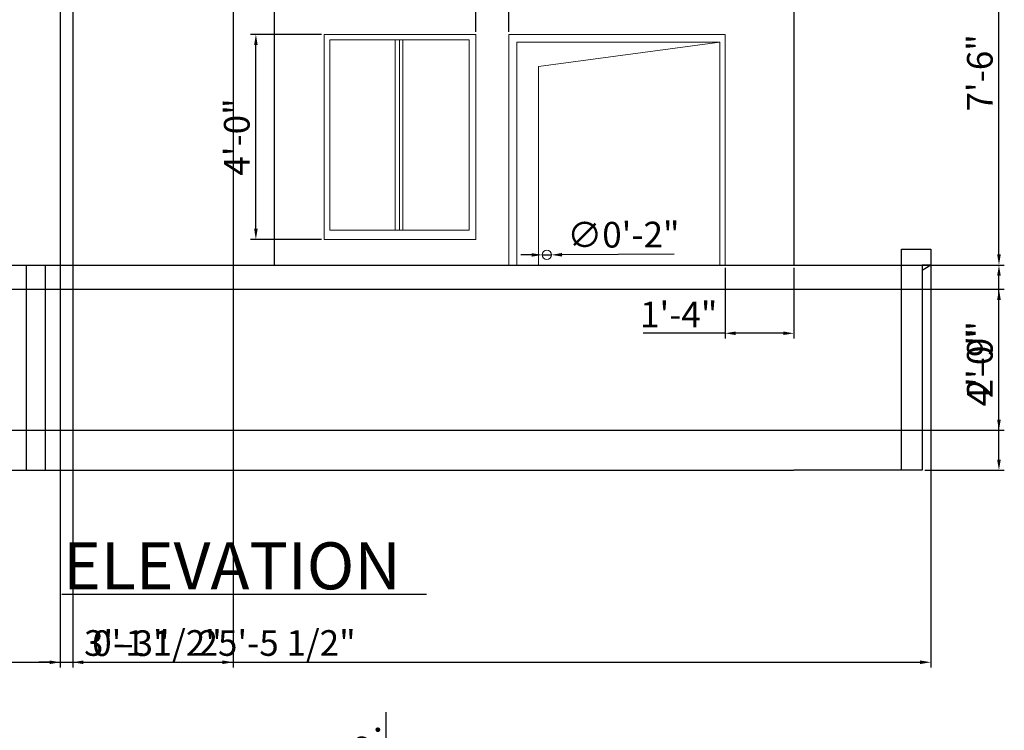
# Model space of a CAD drawing. Units: inches. Extents: x 2656 to 9931, y 1941 to 3068.
# Tile 29 of 46: x 2817 to 3047, y 2689 to 2855. Entities that reach past the tile are written whole.
import ezdxf

# ---------------------------------------------------------------- set-up
doc = ezdxf.new("R2010")
doc.units = ezdxf.units.IN
for name, color, linetype, lineweight in [('A-ANNO-DIMS', 2, 'Continuous', 18), ('A-ANNO-TEXT', 7, 'Continuous', 25), ('A-DOOR', 3, 'Continuous', 18), ('A-ELEV', 7, 'Continuous', 25), ('A-GLAZ', 4, 'Continuous', 18)]:
    doc.layers.add(name, color=color, linetype=linetype, lineweight=lineweight)
doc.styles.get("Standard").update_dxf_attribs({"font": 'arial.ttf'})
doc.dimstyles.new('ISO-25', dxfattribs={"dimtxt": 6, "dimasz": 2.5, "dimexe": 1.25, "dimexo": 0.625, "dimtad": 1, "dimdec": 0, "dimlunit": 3, "dimtxsty": 'Standard', "dimcen": 2.5, "dimadec": 0, "dimazin": 0, "dimtfac": 1, "dimtdec": 0, "dimtmove": 0, "dimatfit": 3, "dimfxl": 1, "dimarcsym": 0})

# ---------------------------------------------------------------- blocks, each defined once
blk = doc.blocks.new('*D33')
at = {"layer": 'A-ANNO-DIMS', "color": 0, "lineweight": -2, "transparency": 16777216}
for p, q in [((2902.86, 2595), (2902.86, 2693.32)), ((2899.03, 2595), (2904.11, 2595)), ((2902.86, 2567.84), (2902.86, 2592.5)), ((2899.03, 2565.34), (2904.11, 2565.34))]:
    blk.add_line(p, q, dxfattribs=at)
at = {"layer": 'A-ANNO-DIMS', "color": 0, "transparency": 16777216}
for points in [[(2902.44, 2592.5), (2903.27, 2592.5), (2902.86, 2595)], [(2902.44, 2567.84), (2903.27, 2567.84), (2902.86, 2565.34)]]:
    blk.add_solid(points, dxfattribs=at)
at = {"layer": 'Defpoints', "color": 0, "transparency": 16777216}
for p in [(2898.41, 2595), (2902.86, 2595), (2898.41, 2565.34)]:
    blk.add_point(p, dxfattribs=at)
at = {"layer": 'A-ANNO-DIMS', "color": 0, "transparency": 16777216, "insert": (2899.13, 2645.41), "char_height": 6, "attachment_point": 5, "rotation": 90}
blk.add_mtext('WC DOOR 2\'-5 1/2" TYP.', dxfattribs=at)
blk = doc.blocks.new('*D63')
at = {"layer": 'A-ANNO-DIMS', "color": 0, "lineweight": -2, "transparency": 16777216}
for p, q in [((2807.09, 2803.32), (2807.09, 2893)), ((2799.7, 2803.32), (2808.34, 2803.32)), ((2807.09, 2752.39), (2807.09, 2800.82)), ((2799.7, 2749.89), (2808.34, 2749.89))]:
    blk.add_line(p, q, dxfattribs=at)
at = {"layer": 'A-ANNO-DIMS', "color": 0, "transparency": 16777216}
for points in [[(2806.67, 2800.82), (2807.5, 2800.82), (2807.09, 2803.32)], [(2806.67, 2752.39), (2807.5, 2752.39), (2807.09, 2749.89)]]:
    blk.add_solid(points, dxfattribs=at)
at = {"layer": 'Defpoints', "color": 0, "transparency": 16777216}
for p in [(2799.07, 2803.32), (2807.09, 2803.32), (2799.07, 2749.89)]:
    blk.add_point(p, dxfattribs=at)
at = {"layer": 'A-ANNO-DIMS', "color": 0, "transparency": 16777216, "insert": (2803.36, 2849.41), "char_height": 6, "attachment_point": 5, "rotation": 90}
blk.add_mtext('FRONT GATE 4\'-5 1/2"', dxfattribs=at)
blk = doc.blocks.new('*D77')
at = {"layer": 'A-ANNO-DIMS', "color": 0, "lineweight": -2, "transparency": 16777216}
for p, q in [((2724.52, 2799.77), (2724.52, 2703.71)), ((3030.16, 2801), (3030.16, 2703.71)), ((2727.02, 2704.96), (3027.66, 2704.96))]:
    blk.add_line(p, q, dxfattribs=at)
at = {"layer": 'A-ANNO-DIMS', "color": 0, "transparency": 16777216}
for points in [[(2727.02, 2705.38), (2727.02, 2704.54), (2724.52, 2704.96)], [(3027.66, 2705.38), (3027.66, 2704.54), (3030.16, 2704.96)]]:
    blk.add_solid(points, dxfattribs=at)
at = {"layer": 'Defpoints', "color": 0, "transparency": 16777216}
for p in [(2724.52, 2800.4), (3030.16, 2801.62), (3030.16, 2704.96)]:
    blk.add_point(p, dxfattribs=at)
at = {"layer": 'A-ANNO-DIMS', "color": 0, "transparency": 16777216, "insert": (2877.34, 2708.69), "char_height": 6, "attachment_point": 5}
blk.add_mtext('25\'-5 1/2"', dxfattribs=at)
blk = doc.blocks.new('*D79')
at = {"layer": 'A-ANNO-DIMS', "color": 0, "lineweight": -2, "transparency": 16777216}
for p, q in [((3023.97, 2797.89), (3047.36, 2797.89)), ((3046.11, 2752.39), (3046.11, 2795.39)), ((3028.78, 2749.89), (3047.36, 2749.89))]:
    blk.add_line(p, q, dxfattribs=at)
at = {"layer": 'A-ANNO-DIMS', "color": 0, "transparency": 16777216}
for points in [[(3045.69, 2795.39), (3046.53, 2795.39), (3046.11, 2797.89)], [(3045.69, 2752.39), (3046.53, 2752.39), (3046.11, 2749.89)]]:
    blk.add_solid(points, dxfattribs=at)
at = {"layer": 'Defpoints', "color": 0, "transparency": 16777216}
for p in [(3023.35, 2797.89), (3046.11, 2797.89), (3028.16, 2749.89)]:
    blk.add_point(p, dxfattribs=at)
at = {"layer": 'A-ANNO-DIMS', "color": 0, "transparency": 16777216, "insert": (3042.42, 2773.89), "char_height": 6, "attachment_point": 5, "rotation": 90}
blk.add_mtext('4\'-0"', dxfattribs=at)
blk = doc.blocks.new('*D80')
at = {"layer": 'A-ANNO-DIMS', "color": 0, "lineweight": -2, "transparency": 16777216}
for p, q in [((3015.61, 2887.89), (3047.36, 2887.89)), ((3046.11, 2800.39), (3046.11, 2885.39)), ((2998.78, 2797.89), (3047.36, 2797.89))]:
    blk.add_line(p, q, dxfattribs=at)
at = {"layer": 'A-ANNO-DIMS', "color": 0, "transparency": 16777216}
for points in [[(3045.69, 2885.39), (3046.53, 2885.39), (3046.11, 2887.89)], [(3045.69, 2800.39), (3046.53, 2800.39), (3046.11, 2797.89)]]:
    blk.add_solid(points, dxfattribs=at)
at = {"layer": 'Defpoints', "color": 0, "transparency": 16777216}
for p in [(3014.98, 2887.89), (3046.11, 2887.89), (2998.16, 2797.89)]:
    blk.add_point(p, dxfattribs=at)
at = {"layer": 'A-ANNO-DIMS', "color": 0, "transparency": 16777216, "insert": (3042.42, 2842.89), "char_height": 6, "attachment_point": 5, "rotation": 90}
blk.add_mtext('7\'-6"', dxfattribs=at)
blk = doc.blocks.new('*D82')
at = {"layer": 'A-ANNO-DIMS', "color": 0, "lineweight": -2, "transparency": 16777216}
for p, q in [((2887.7, 2851.89), (2871.12, 2851.89)), ((2872.37, 2806.39), (2872.37, 2849.39)), ((2887.7, 2803.89), (2871.12, 2803.89))]:
    blk.add_line(p, q, dxfattribs=at)
at = {"layer": 'A-ANNO-DIMS', "color": 0, "transparency": 16777216}
for points in [[(2871.96, 2849.39), (2872.79, 2849.39), (2872.37, 2851.89)], [(2871.96, 2806.39), (2872.79, 2806.39), (2872.37, 2803.89)]]:
    blk.add_solid(points, dxfattribs=at)
at = {"layer": 'Defpoints', "color": 0, "transparency": 16777216}
for p in [(2872.37, 2851.89), (2888.32, 2851.89), (2888.32, 2803.89)]:
    blk.add_point(p, dxfattribs=at)
at = {"layer": 'A-ANNO-DIMS', "color": 0, "transparency": 16777216, "insert": (2868.68, 2827.89), "char_height": 6, "attachment_point": 5, "rotation": 90}
blk.add_mtext('4\'-0"', dxfattribs=at)
blk = doc.blocks.new('*D86')
at = {"layer": 'A-ANNO-DIMS', "color": 0, "lineweight": -2, "transparency": 16777216}
for p, q in [((2923.8, 2852.52), (2923.8, 2869.09)), ((2931.54, 2852.52), (2931.54, 2869.09)), ((2926.3, 2867.84), (2929.04, 2867.84)), ((2931.54, 2867.84), (2965.22, 2867.84))]:
    blk.add_line(p, q, dxfattribs=at)
at = {"layer": 'A-ANNO-DIMS', "color": 0, "transparency": 16777216}
for points in [[(2926.3, 2868.26), (2926.3, 2867.43), (2923.8, 2867.84)], [(2929.04, 2868.26), (2929.04, 2867.43), (2931.54, 2867.84)]]:
    blk.add_solid(points, dxfattribs=at)
at = {"layer": 'Defpoints', "color": 0, "transparency": 16777216}
for p in [(2931.54, 2867.84), (2923.8, 2851.89), (2931.54, 2851.89)]:
    blk.add_point(p, dxfattribs=at)
at = {"layer": 'A-ANNO-DIMS', "color": 0, "transparency": 16777216, "insert": (2949.63, 2871.57), "char_height": 6, "attachment_point": 5}
blk.add_mtext('0\'-7 1/2"', dxfattribs=at)
blk = doc.blocks.new('*D87')
at = {"layer": 'A-ANNO-DIMS', "color": 0, "lineweight": -2, "transparency": 16777216}
for p, q in [((2982.06, 2797.27), (2982.06, 2780.69)), ((2998.16, 2797.27), (2998.16, 2780.69)), ((2982.06, 2781.94), (2962.92, 2781.94)), ((2995.66, 2781.94), (2984.56, 2781.94))]:
    blk.add_line(p, q, dxfattribs=at)
at = {"layer": 'A-ANNO-DIMS', "color": 0, "transparency": 16777216}
for points in [[(2984.56, 2782.36), (2984.56, 2781.53), (2982.06, 2781.94)], [(2995.66, 2782.36), (2995.66, 2781.53), (2998.16, 2781.94)]]:
    blk.add_solid(points, dxfattribs=at)
at = {"layer": 'Defpoints', "color": 0, "transparency": 16777216}
for p in [(2982.06, 2797.89), (2998.16, 2797.89), (2982.06, 2781.94)]:
    blk.add_point(p, dxfattribs=at)
at = {"layer": 'A-ANNO-DIMS', "color": 0, "transparency": 16777216, "insert": (2971.24, 2785.58), "char_height": 6, "attachment_point": 5}
blk.add_mtext('1\'-4"', dxfattribs=at)
blk = doc.blocks.new('*D151')
at = {"layer": 'A-ANNO-DIMS', "color": 0, "lineweight": -2, "transparency": 16777216}
for p, q in [((2829.55, 2956.42), (2829.55, 2703.71)), ((2867.06, 2955.98), (2867.06, 2703.71)), ((2832.05, 2704.96), (2864.56, 2704.96))]:
    blk.add_line(p, q, dxfattribs=at)
at = {"layer": 'A-ANNO-DIMS', "color": 0, "transparency": 16777216}
for points in [[(2832.05, 2705.38), (2832.05, 2704.54), (2829.55, 2704.96)], [(2864.56, 2705.38), (2864.56, 2704.54), (2867.06, 2704.96)]]:
    blk.add_solid(points, dxfattribs=at)
at = {"layer": 'Defpoints', "color": 0, "transparency": 16777216}
for p in [(2829.55, 2957.05), (2867.06, 2956.61), (2867.06, 2704.96)]:
    blk.add_point(p, dxfattribs=at)
at = {"layer": 'A-ANNO-DIMS', "color": 0, "transparency": 16777216, "insert": (2848.3, 2708.69), "char_height": 6, "attachment_point": 5}
blk.add_mtext('3\'-1 1/2"', dxfattribs=at)
blk = doc.blocks.new('*D153')
at = {"layer": 'A-ANNO-DIMS', "color": 0, "lineweight": -2, "transparency": 16777216}
for p, q in [((2826.64, 2993.72), (2826.64, 2703.71)), ((2829.55, 2956.42), (2829.55, 2703.71)), ((2824.14, 2704.96), (2821.64, 2704.96)), ((2826.64, 2704.96), (2829.55, 2704.96)), ((2832.05, 2704.96), (2851.75, 2704.96))]:
    blk.add_line(p, q, dxfattribs=at)
at = {"layer": 'A-ANNO-DIMS', "color": 0, "transparency": 16777216}
for points in [[(2824.14, 2705.38), (2824.14, 2704.54), (2826.64, 2704.96)], [(2832.05, 2705.38), (2832.05, 2704.54), (2829.55, 2704.96)]]:
    blk.add_solid(points, dxfattribs=at)
at = {"layer": 'Defpoints', "color": 0, "transparency": 16777216}
for p in [(2826.64, 2994.35), (2829.55, 2957.05), (2829.55, 2704.96)]:
    blk.add_point(p, dxfattribs=at)
at = {"layer": 'A-ANNO-DIMS', "color": 0, "transparency": 16777216, "insert": (2843.15, 2708.65), "char_height": 6, "attachment_point": 5}
blk.add_mtext('0\'-3"', dxfattribs=at)
blk = doc.blocks.new('*D179')
at = {"layer": 'A-ANNO-DIMS', "color": 0, "lineweight": -2, "transparency": 16777216}
for p, q in [((2772.12, 2792.27), (3047.36, 2792.27)), ((3046.11, 2761.76), (3046.11, 2789.77)), ((2772.31, 2759.26), (3047.36, 2759.26))]:
    blk.add_line(p, q, dxfattribs=at)
at = {"layer": 'A-ANNO-DIMS', "color": 0, "transparency": 16777216}
for points in [[(3045.69, 2789.77), (3046.53, 2789.77), (3046.11, 2792.27)], [(3045.69, 2761.76), (3046.53, 2761.76), (3046.11, 2759.26)]]:
    blk.add_solid(points, dxfattribs=at)
at = {"layer": 'Defpoints', "color": 0, "transparency": 16777216}
for p in [(2771.5, 2792.27), (3046.11, 2792.27), (2771.68, 2759.26)]:
    blk.add_point(p, dxfattribs=at)
at = {"layer": 'A-ANNO-DIMS', "color": 0, "transparency": 16777216, "insert": (3042.42, 2775.76), "char_height": 6, "attachment_point": 5, "rotation": 90}
blk.add_mtext('2\'-9"', dxfattribs=at)
blk = doc.blocks.new('*D195')
at = {"layer": 'A-ANNO-DIMS', "color": 0, "lineweight": -2, "transparency": 16777216}
for p, q in [((2936.83, 2800.28), (2934.33, 2800.27)), ((2939.33, 2800.29), (2941.47, 2800.3)), ((2970.19, 2800.44), (2943.97, 2800.31))]:
    blk.add_line(p, q, dxfattribs=at)
at = {"layer": 'A-ANNO-DIMS', "color": 0, "transparency": 16777216}
for points in [[(2936.83, 2800.69), (2936.83, 2799.86), (2939.33, 2800.29)], [(2943.96, 2800.73), (2943.97, 2799.89), (2941.47, 2800.3)]]:
    blk.add_solid(points, dxfattribs=at)
at = {"layer": 'Defpoints', "color": 0, "transparency": 16777216}
for p in [(2939.33, 2800.29), (2941.47, 2800.3)]:
    blk.add_point(p, dxfattribs=at)
at = {"layer": 'A-ANNO-DIMS', "color": 0, "transparency": 16777216, "insert": (2958.31, 2804.24), "char_height": 6, "attachment_point": 5, "rotation": 0.2723}
blk.add_mtext('∅0\'-2"', dxfattribs=at)

msp = doc.modelspace()

# ---------------------------------------------------------------- linework, layer by layer
at = {"layer": 'A-ANNO-TEXT'}
msp.add_line((2827.02, 2720.91), (2912.29, 2720.91), dxfattribs=at)
at = {"layer": 'A-DOOR'}
for p, q in [((2982.06, 2851.89), (2931.54, 2851.89)), ((2931.54, 2851.89), (2931.54, 2797.89)), ((2980.83, 2850.05), (2938.49, 2844.38)), ((2982.06, 2851.89), (2982.06, 2797.89)), ((2938.49, 2844.38), (2938.49, 2797.89))]:
    msp.add_line(p, q, dxfattribs=at)
for points in [[(2931.54, 2797.89), (2931.54, 2851.89), (2982.06, 2851.89), (2982.06, 2797.89)], [(2933.35, 2797.89), (2933.35, 2850.05), (2980.83, 2850.05), (2980.83, 2797.89)]]:
    msp.add_lwpolyline(points, dxfattribs=at)
msp.add_circle((2940.4, 2800.29), 1.07, dxfattribs=at)
at = {"layer": 'A-ELEV'}
for p, q in [((2876.66, 2887.89), (2876.66, 2797.89)), ((2998.16, 2887.89), (2998.16, 2797.89)), ((3023.35, 2749.89), (3023.35, 2801.62)), ((3023.35, 2801.62), (3023.35, 2801.62)), ((3023.35, 2801.62), (3030.16, 2801.62)), ((3030.16, 2801.62), (3030.16, 2798.02)), ((2796.75, 2797.89), (3023.35, 2797.89)), ((2818.67, 2797.89), (2818.67, 2749.89)), ((2823.18, 2749.89), (2823.18, 2797.89)), ((3028.16, 2797.89), (3028.16, 2749.89)), ((3030.16, 2797.89), (3028.16, 2797.89)), ((3030.16, 2797.89), (3028.16, 2796.62)), ((3030.16, 2798.02), (3030.16, 2797.89)), ((2743.16, 2749.89), (2998.16, 2749.89)), ((2743.16, 2749.89), (2998.16, 2749.89)), ((2818.67, 2749.89), (2823.18, 2749.89)), ((3028.16, 2749.89), (2998.16, 2749.89)), ((3028.16, 2749.89), (3023.35, 2749.89)), ((3028.16, 2749.89), (3028.16, 2749.89))]:
    msp.add_line(p, q, dxfattribs=at)
at = {"layer": 'A-GLAZ'}
for p, q in [((2888.32, 2851.89), (2888.32, 2803.89)), ((2923.8, 2851.89), (2888.32, 2851.89)), ((2905.94, 2850.62), (2904.94, 2850.62)), ((2904.94, 2850.62), (2904.94, 2806.06)), ((2905.94, 2850.62), (2905.94, 2806.06)), ((2906.75, 2806.06), (2906.75, 2850.62)), ((2923.8, 2851.89), (2923.8, 2803.89)), ((2904.94, 2806.06), (2906.75, 2806.06)), ((2923.8, 2803.89), (2888.32, 2803.89))]:
    msp.add_line(p, q, dxfattribs=at)
for points in [[(2888.32, 2851.89), (2923.8, 2851.89), (2923.8, 2803.89), (2888.32, 2803.89)], [(2889.68, 2850.62), (2922.21, 2850.62), (2922.21, 2806.06), (2889.68, 2806.06)]]:
    msp.add_lwpolyline(points, close=True, dxfattribs=at)

# ---------------------------------------------------------------- texts
at = {"layer": 'A-ANNO-TEXT', "insert": (2827.3, 2733.02), "char_height": 11, "attachment_point": 1}
msp.add_mtext_dynamic_manual_height_columns('ELEVATION', width=308.3307, gutter_width=12.5, heights=[0], dxfattribs=at)

# ---------------------------------------------------------------- dimensions: what is measured, and where the dimension line sits
at = {"layer": 'A-ANNO-DIMS'}
for base, p1, p2, picture, middle in [((2829.55, 2704.96), (2826.64, 2994.35), (2829.55, 2957.05), '*D153', (2843.15, 2708.65)), ((2867.06, 2704.96), (2829.55, 2957.05), (2867.06, 2956.61), '*D151', (2848.3, 2708.69)), ((2931.54, 2867.84), (2923.8, 2851.89), (2931.54, 2851.89), '*D86', (2949.63, 2871.57)), ((3030.16, 2704.96), (2724.52, 2800.4), (3030.16, 2801.62), '*D77', (2877.34, 2708.69))]:
    dim = msp.add_linear_dim(base=base, p1=p1, p2=p2, dimstyle='ISO-25', override={"dimdec": 1, "dimlfac": 1, "dimrnd": 0, "dimzin": 1, "dimdsep": 46, "dimlunit": 4, "dimfrac": 2}, dxfattribs=at)
    dim.commit()
    dim.dimension.update_dxf_attribs({"geometry": picture, "text_midpoint": middle})
for base, p1, p2, text, picture, middle in [((2807.09, 2803.32), (2799.07, 2749.89), (2799.07, 2803.32), 'FRONT GATE <>', '*D63', (2803.36, 2849.41)), ((2902.86, 2595), (2898.41, 2565.34), (2898.41, 2595), 'WC DOOR <> TYP.', '*D33', (2899.13, 2645.41))]:
    dim = msp.add_linear_dim(base=base, p1=p1, p2=p2, angle=90, text=text, dimstyle='ISO-25', override={"dimdec": 1, "dimlfac": 1, "dimrnd": 0, "dimzin": 1, "dimdsep": 46, "dimlunit": 4, "dimfrac": 2}, dxfattribs=at)
    dim.commit()
    dim.dimension.update_dxf_attribs({"geometry": picture, "text_midpoint": middle})
for base, p1, p2, angle, picture, middle in [((3046.11, 2887.89), (2998.16, 2797.89), (3014.98, 2887.89), 90, '*D80', (3042.42, 2842.89)), ((2872.37, 2851.89), (2888.32, 2803.89), (2888.32, 2851.89), 90, '*D82', (2868.68, 2827.89)), ((2982.06, 2781.94), (2998.16, 2797.89), (2982.06, 2797.89), 180, '*D87', (2971.24, 2785.58)), ((3046.11, 2797.89), (3028.16, 2749.89), (3023.35, 2797.89), 90, '*D79', (3042.42, 2773.89)), ((3046.11, 2792.27), (2771.68, 2759.26), (2771.5, 2792.27), 90, '*D179', (3042.42, 2775.76))]:
    dim = msp.add_linear_dim(base=base, p1=p1, p2=p2, angle=angle, dimstyle='ISO-25', override={"dimdec": 1, "dimlfac": 1, "dimrnd": 0, "dimzin": 1, "dimdsep": 46, "dimlunit": 4, "dimfrac": 2}, dxfattribs=at)
    dim.commit()
    dim.dimension.update_dxf_attribs({"geometry": picture, "text_midpoint": middle})
dim = msp.add_diameter_dim_2p(p1=(2939.33, 2800.29), p2=(2941.47, 2800.3), dimstyle='ISO-25', override={"dimdec": 1, "dimlfac": 1, "dimrnd": 0, "dimzin": 1, "dimdsep": 46, "dimlunit": 4, "dimfrac": 2}, dxfattribs=at)
dim.commit()
dim.dimension.update_dxf_attribs({"geometry": '*D195', "text_midpoint": (2958.33, 2800.38), "dimtype": 163})

doc.saveas('drawing.dxf')
